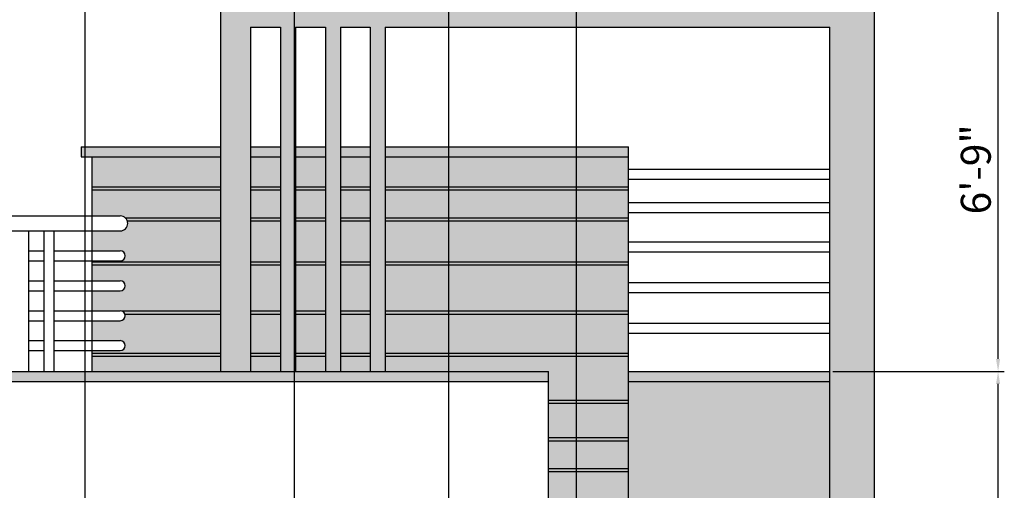
# Model space of a CAD drawing. Units: millimetres. Extents: x 4237 to 5109, y 21391 to 22486.
# Tile 4 of 17: x 4911 to 5109, y 21704 to 21798. Entities that reach past the tile are written whole.
import ezdxf

# ---------------------------------------------------------------- set-up
doc = ezdxf.new("R2010")
doc.units = ezdxf.units.MM
for name, color, linetype, lineweight in [('A-ANNO-DIMS', 2, 'Continuous', 18), ('A-ELEV', 7, 'Continuous', 25), ('A-ELEV-PATT', 252, 'Continuous', 13)]:
    doc.layers.add(name, color=color, linetype=linetype, lineweight=lineweight)
doc.styles.get("Standard").update_dxf_attribs({"font": 'arial.ttf'})
doc.dimstyles.new('ISO-25', dxfattribs={"dimtxt": 6, "dimasz": 2.5, "dimexe": 1.25, "dimexo": 0.625, "dimtad": 1, "dimdec": 1, "dimlunit": 4, "dimtxsty": 'Standard', "dimcen": 2.5, "dimadec": 0, "dimazin": 0, "dimtfac": 1, "dimtdec": 1, "dimtmove": 0, "dimatfit": 3, "dimfxl": 1, "dimarcsym": 0})

# ---------------------------------------------------------------- blocks, each defined once
blk = doc.blocks.new('*D130')
at = {"layer": 'A-ANNO-DIMS', "color": 0, "lineweight": -2, "transparency": 16777216}
for p, q in [((4878.54, 21688.54), (4878.54, 21897.84)), ((4881.04, 21896.59), (4921.78, 21896.59)), ((4924.28, 21686.68), (4924.28, 21897.84))]:
    blk.add_line(p, q, dxfattribs=at)
at = {"layer": 'A-ANNO-DIMS', "color": 0, "transparency": 16777216}
for points in [[(4881.04, 21897), (4881.04, 21896.17), (4878.54, 21896.59)], [(4921.78, 21897), (4921.78, 21896.17), (4924.28, 21896.59)]]:
    blk.add_solid(points, dxfattribs=at)
at = {"layer": 'Defpoints', "color": 0, "transparency": 16777216}
for p in [(4924.28, 21896.59), (4878.54, 21687.91), (4924.28, 21686.05)]:
    blk.add_point(p, dxfattribs=at)
at = {"layer": 'A-ANNO-DIMS', "color": 0, "transparency": 16777216, "insert": (4901.41, 21900.32), "char_height": 6, "attachment_point": 5}
blk.add_mtext('3\'-9 1/2"', dxfattribs=at)
blk = doc.blocks.new('*D131')
at = {"layer": 'A-ANNO-DIMS', "color": 0, "lineweight": -2, "transparency": 16777216}
for p, q in [((4924.28, 21686.68), (4924.28, 21897.84)), ((4926.78, 21896.59), (4963.73, 21896.59)), ((4966.23, 21686.68), (4966.23, 21897.84))]:
    blk.add_line(p, q, dxfattribs=at)
at = {"layer": 'A-ANNO-DIMS', "color": 0, "transparency": 16777216}
for points in [[(4926.78, 21897), (4926.78, 21896.17), (4924.28, 21896.59)], [(4963.73, 21897), (4963.73, 21896.17), (4966.23, 21896.59)]]:
    blk.add_solid(points, dxfattribs=at)
at = {"layer": 'Defpoints', "color": 0, "transparency": 16777216}
for p in [(4966.23, 21896.59), (4924.28, 21686.05), (4966.23, 21686.05)]:
    blk.add_point(p, dxfattribs=at)
at = {"layer": 'A-ANNO-DIMS', "color": 0, "transparency": 16777216, "insert": (4945.25, 21900.28), "char_height": 6, "attachment_point": 5}
blk.add_mtext('3\'-6"', dxfattribs=at)
blk = doc.blocks.new('*D132')
at = {"layer": 'A-ANNO-DIMS', "color": 0, "lineweight": -2, "transparency": 16777216}
for p, q in [((4966.23, 21686.68), (4966.23, 21897.84)), ((4968.73, 21896.59), (4994.7, 21896.59)), ((4997.2, 21689.78), (4997.2, 21897.84))]:
    blk.add_line(p, q, dxfattribs=at)
at = {"layer": 'A-ANNO-DIMS', "color": 0, "transparency": 16777216}
for points in [[(4968.73, 21897), (4968.73, 21896.17), (4966.23, 21896.59)], [(4994.7, 21897), (4994.7, 21896.17), (4997.2, 21896.59)]]:
    blk.add_solid(points, dxfattribs=at)
at = {"layer": 'Defpoints', "color": 0, "transparency": 16777216}
for p in [(4997.2, 21896.59), (4997.2, 21689.16), (4966.23, 21686.05)]:
    blk.add_point(p, dxfattribs=at)
at = {"layer": 'A-ANNO-DIMS', "color": 0, "transparency": 16777216, "insert": (4981.72, 21900.22), "char_height": 6, "attachment_point": 5}
blk.add_mtext('2\'-7"', dxfattribs=at)
blk = doc.blocks.new('*D133')
at = {"layer": 'A-ANNO-DIMS', "color": 0, "lineweight": -2, "transparency": 16777216}
for p, q in [((4997.2, 21689.78), (4997.2, 21897.84)), ((4999.7, 21896.59), (5020.26, 21896.59)), ((5022.76, 21689.78), (5022.76, 21897.84)), ((5022.76, 21896.59), (5056.55, 21896.59))]:
    blk.add_line(p, q, dxfattribs=at)
at = {"layer": 'A-ANNO-DIMS', "color": 0, "transparency": 16777216}
for points in [[(4999.7, 21897), (4999.7, 21896.17), (4997.2, 21896.59)], [(5020.26, 21897), (5020.26, 21896.17), (5022.76, 21896.59)]]:
    blk.add_solid(points, dxfattribs=at)
at = {"layer": 'Defpoints', "color": 0, "transparency": 16777216}
for p in [(5022.76, 21896.59), (4997.2, 21689.16), (5022.76, 21689.16)]:
    blk.add_point(p, dxfattribs=at)
at = {"layer": 'A-ANNO-DIMS', "color": 0, "transparency": 16777216, "insert": (5040.91, 21900.31), "char_height": 6, "attachment_point": 5}
blk.add_mtext('2\'-1 1/2"', dxfattribs=at)
blk = doc.blocks.new('*D134')
at = {"layer": 'A-ANNO-DIMS', "color": 0, "lineweight": -2, "transparency": 16777216}
for p, q in [((5022.76, 21689.78), (5022.76, 21897.84)), ((5025.26, 21896.59), (5080.03, 21896.59)), ((5082.53, 21809.46), (5082.53, 21897.84))]:
    blk.add_line(p, q, dxfattribs=at)
at = {"layer": 'A-ANNO-DIMS', "color": 0, "transparency": 16777216}
for points in [[(5025.26, 21897), (5025.26, 21896.17), (5022.76, 21896.59)], [(5080.03, 21897), (5080.03, 21896.17), (5082.53, 21896.59)]]:
    blk.add_solid(points, dxfattribs=at)
at = {"layer": 'Defpoints', "color": 0, "transparency": 16777216}
for p in [(5082.53, 21896.59), (5082.53, 21808.84), (5022.76, 21689.16)]:
    blk.add_point(p, dxfattribs=at)
at = {"layer": 'A-ANNO-DIMS', "color": 0, "transparency": 16777216, "insert": (5052.65, 21900.27), "char_height": 6, "attachment_point": 5}
blk.add_mtext('5\'-0"', dxfattribs=at)
blk = doc.blocks.new('*D136')
at = {"layer": 'A-ANNO-DIMS', "color": 0, "lineweight": -2, "transparency": 16777216}
for p, q in [((5074.15, 21727.84), (5108.53, 21727.84)), ((5107.28, 21560.34), (5107.28, 21725.34)), ((5083.15, 21557.84), (5108.53, 21557.84))]:
    blk.add_line(p, q, dxfattribs=at)
at = {"layer": 'A-ANNO-DIMS', "color": 0, "transparency": 16777216}
for points in [[(5106.86, 21725.34), (5107.69, 21725.34), (5107.28, 21727.84)], [(5106.86, 21560.34), (5107.69, 21560.34), (5107.28, 21557.84)]]:
    blk.add_solid(points, dxfattribs=at)
at = {"layer": 'Defpoints', "color": 0, "transparency": 16777216}
for p in [(5073.53, 21727.84), (5107.28, 21727.84), (5082.53, 21557.84)]:
    blk.add_point(p, dxfattribs=at)
at = {"layer": 'A-ANNO-DIMS', "color": 0, "transparency": 16777216, "insert": (5103.64, 21642.84), "char_height": 6, "attachment_point": 5, "rotation": 90}
blk.add_mtext('14\'-2"', dxfattribs=at)
blk = doc.blocks.new('*D137')
at = {"layer": 'A-ANNO-DIMS', "color": 0, "lineweight": -2, "transparency": 16777216}
for p, q in [((5083.15, 21808.84), (5108.53, 21808.84)), ((5107.28, 21730.34), (5107.28, 21806.34)), ((5074.15, 21727.84), (5108.53, 21727.84))]:
    blk.add_line(p, q, dxfattribs=at)
at = {"layer": 'A-ANNO-DIMS', "color": 0, "transparency": 16777216}
for points in [[(5106.86, 21806.34), (5107.69, 21806.34), (5107.28, 21808.84)], [(5106.86, 21730.34), (5107.69, 21730.34), (5107.28, 21727.84)]]:
    blk.add_solid(points, dxfattribs=at)
at = {"layer": 'Defpoints', "color": 0, "transparency": 16777216}
for p in [(5082.53, 21808.84), (5107.28, 21808.84), (5073.53, 21727.84)]:
    blk.add_point(p, dxfattribs=at)
at = {"layer": 'A-ANNO-DIMS', "color": 0, "transparency": 16777216, "insert": (5103.59, 21768.34), "char_height": 6, "attachment_point": 5, "rotation": 90}
blk.add_mtext('6\'-9"', dxfattribs=at)

msp = doc.modelspace()

# ---------------------------------------------------------------- hatches: boundary and pattern name
at = {"layer": 'A-ELEV-PATT'}
h = msp.add_hatch(color=256, dxfattribs=at)
h.dxf.hatch_style = 1
h.paths.add_polyline_path([(4957.45, 21796.84), (4963.45, 21796.84), (4963.45, 21727.84), (4966.45, 21727.84), (4966.45, 21796.84), (4972.45, 21796.84), (4972.45, 21727.84), (4975.45, 21727.84), (4975.45, 21796.84), (4981.45, 21796.84), (4981.45, 21727.84), (4984.45, 21727.84), (4984.45, 21796.84), (5073.53, 21796.84), (5073.53, 21557.84), (5082.53, 21557.84), (5082.53, 21808.84), (4951.45, 21808.84), (4951.45, 21727.84), (4957.45, 21727.84)])
h = msp.add_hatch(color=256, dxfattribs=at)
h.dxf.hatch_style = 1
h.paths.add_polyline_path([(4951.45, 21772.84), (4923.48, 21772.84), (4923.48, 21770.84), (4951.45, 21770.84)])
h = msp.add_hatch(color=256, dxfattribs=at)
h.dxf.hatch_style = 1
h.paths.add_polyline_path([(4963.45, 21772.84), (4957.45, 21772.84), (4957.45, 21770.84), (4963.45, 21770.84)])
h = msp.add_hatch(color=256, dxfattribs=at)
h.dxf.hatch_style = 1
h.paths.add_polyline_path([(4972.45, 21772.84), (4966.45, 21772.84), (4966.45, 21770.84), (4972.45, 21770.84)])
h = msp.add_hatch(color=256, dxfattribs=at)
h.dxf.hatch_style = 1
h.paths.add_polyline_path([(4981.45, 21772.84), (4975.45, 21772.84), (4975.45, 21770.84), (4981.45, 21770.84)])
h = msp.add_hatch(color=256, dxfattribs=at)
h.dxf.hatch_style = 1
h.paths.add_polyline_path([(5033.17, 21772.84), (4984.45, 21772.84), (4984.45, 21770.84), (5033.17, 21770.84)])
h = msp.add_hatch(color=256, dxfattribs=at)
h.dxf.hatch_style = 1
h.paths.add_polyline_path([(4951.45, 21770.84), (4925.69, 21770.84), (4925.69, 21764.85), (4951.45, 21764.85)])
h = msp.add_hatch(color=256, dxfattribs=at)
h.dxf.hatch_style = 1
h.paths.add_polyline_path([(4963.45, 21770.84), (4957.45, 21770.84), (4957.45, 21764.85), (4963.45, 21764.85)])
h = msp.add_hatch(color=256, dxfattribs=at)
h.dxf.hatch_style = 1
h.paths.add_polyline_path([(4972.45, 21770.84), (4966.45, 21770.84), (4966.45, 21764.85), (4972.45, 21764.85)])
h = msp.add_hatch(color=256, dxfattribs=at)
h.dxf.hatch_style = 1
h.paths.add_polyline_path([(4981.45, 21770.84), (4975.45, 21770.84), (4975.45, 21764.85), (4981.45, 21764.85)])
h = msp.add_hatch(color=256, dxfattribs=at)
h.dxf.hatch_style = 1
h.paths.add_polyline_path([(5033.17, 21770.84), (4984.45, 21770.84), (4984.45, 21764.85), (5033.17, 21764.85)])
h = msp.add_hatch(color=256, dxfattribs=at)
h.dxf.hatch_style = 1
h.paths.add_polyline_path([(4951.45, 21764.85), (4925.69, 21764.85), (4925.69, 21764.23), (4951.45, 21764.23)])
h = msp.add_hatch(color=256, dxfattribs=at)
h.dxf.hatch_style = 1
h.paths.add_polyline_path([(4951.45, 21764.23), (4925.69, 21764.23), (4925.69, 21759.01), (4931.32, 21759.01, -0.184847), (4932.32, 21758.63), (4951.45, 21758.63)])
h = msp.add_hatch(color=256, dxfattribs=at)
h.dxf.hatch_style = 1
h.paths.add_polyline_path([(4963.45, 21764.85), (4957.45, 21764.85), (4957.45, 21764.23), (4963.45, 21764.23)])
h = msp.add_hatch(color=256, dxfattribs=at)
h.dxf.hatch_style = 1
h.paths.add_polyline_path([(4963.45, 21764.23), (4957.45, 21764.23), (4957.45, 21758.63), (4963.45, 21758.63)])
h = msp.add_hatch(color=256, dxfattribs=at)
h.dxf.hatch_style = 1
h.paths.add_polyline_path([(4972.45, 21764.85), (4966.45, 21764.85), (4966.45, 21764.23), (4972.45, 21764.23)])
h = msp.add_hatch(color=256, dxfattribs=at)
h.dxf.hatch_style = 1
h.paths.add_polyline_path([(4972.45, 21764.23), (4966.45, 21764.23), (4966.45, 21758.63), (4972.45, 21758.63)])
h = msp.add_hatch(color=256, dxfattribs=at)
h.dxf.hatch_style = 1
h.paths.add_polyline_path([(4981.45, 21764.85), (4975.45, 21764.85), (4975.45, 21764.23), (4981.45, 21764.23)])
h = msp.add_hatch(color=256, dxfattribs=at)
h.dxf.hatch_style = 1
h.paths.add_polyline_path([(4981.45, 21764.23), (4975.45, 21764.23), (4975.45, 21758.63), (4981.45, 21758.63)])
h = msp.add_hatch(color=256, dxfattribs=at)
h.dxf.hatch_style = 1
h.paths.add_polyline_path([(5033.17, 21764.85), (4984.45, 21764.85), (4984.45, 21764.23), (5033.17, 21764.23)])
h = msp.add_hatch(color=256, dxfattribs=at)
h.dxf.hatch_style = 1
h.paths.add_polyline_path([(5033.17, 21764.23), (4984.45, 21764.23), (4984.45, 21758.63), (5033.17, 21758.63)])
h = msp.add_hatch(color=256, dxfattribs=at)
h.dxf.hatch_style = 1
h.paths.add_polyline_path([(4951.45, 21758.63), (4932.32, 21758.63, -0.127629), (4932.74, 21758), (4951.45, 21758)])
h = msp.add_hatch(color=256, dxfattribs=at)
h.dxf.hatch_style = 1
h.paths.add_polyline_path([(4963.45, 21758.63), (4957.45, 21758.63), (4957.45, 21758), (4963.45, 21758)])
h = msp.add_hatch(color=256, dxfattribs=at)
h.dxf.hatch_style = 1
h.paths.add_polyline_path([(4972.45, 21758.63), (4966.45, 21758.63), (4966.45, 21758), (4972.45, 21758)])
h = msp.add_hatch(color=256, dxfattribs=at)
h.dxf.hatch_style = 1
h.paths.add_polyline_path([(4981.45, 21758.63), (4975.45, 21758.63), (4975.45, 21758), (4981.45, 21758)])
h = msp.add_hatch(color=256, dxfattribs=at)
h.dxf.hatch_style = 1
h.paths.add_polyline_path([(5033.17, 21758.63), (4984.45, 21758.63), (4984.45, 21758), (5033.17, 21758)])
h = msp.add_hatch(color=256, dxfattribs=at)
h.dxf.hatch_style = 1
h.paths.add_polyline_path([(4951.45, 21758), (4932.74, 21758, -0.515121), (4931.32, 21756.01), (4925.69, 21756.01), (4925.69, 21752.01), (4931.32, 21752.01, -1), (4931.32, 21750.01), (4925.69, 21750.01), (4925.69, 21749.81), (4951.45, 21749.81)])
h = msp.add_hatch(color=256, dxfattribs=at)
h.dxf.hatch_style = 1
h.paths.add_polyline_path([(4963.45, 21758), (4957.45, 21758), (4957.45, 21749.81), (4963.45, 21749.81)])
h = msp.add_hatch(color=256, dxfattribs=at)
h.dxf.hatch_style = 1
h.paths.add_polyline_path([(4972.45, 21758), (4966.45, 21758), (4966.45, 21749.81), (4972.45, 21749.81)])
h = msp.add_hatch(color=256, dxfattribs=at)
h.dxf.hatch_style = 1
h.paths.add_polyline_path([(4981.45, 21758), (4975.45, 21758), (4975.45, 21749.81), (4981.45, 21749.81)])
h = msp.add_hatch(color=256, dxfattribs=at)
h.dxf.hatch_style = 1
h.paths.add_polyline_path([(5033.17, 21758), (4984.45, 21758), (4984.45, 21749.81), (5033.17, 21749.81)])
h = msp.add_hatch(color=256, dxfattribs=at)
h.dxf.hatch_style = 1
h.paths.add_polyline_path([(4951.45, 21749.81), (4925.69, 21749.81), (4925.69, 21749.18), (4951.45, 21749.18)])
h = msp.add_hatch(color=256, dxfattribs=at)
h.dxf.hatch_style = 1
h.paths.add_polyline_path([(4951.45, 21749.18), (4925.69, 21749.18), (4925.69, 21746.01), (4931.32, 21746.01, -1), (4931.32, 21744.01), (4925.69, 21744.01), (4925.69, 21740.01), (4931.32, 21740.01, -0.068465), (4931.59, 21739.97), (4951.45, 21739.97)])
h = msp.add_hatch(color=256, dxfattribs=at)
h.dxf.hatch_style = 1
h.paths.add_polyline_path([(4963.45, 21749.81), (4957.45, 21749.81), (4957.45, 21749.18), (4963.45, 21749.18)])
h = msp.add_hatch(color=256, dxfattribs=at)
h.dxf.hatch_style = 1
h.paths.add_polyline_path([(4963.45, 21749.18), (4957.45, 21749.18), (4957.45, 21739.97), (4963.45, 21739.97)])
h = msp.add_hatch(color=256, dxfattribs=at)
h.dxf.hatch_style = 1
h.paths.add_polyline_path([(4972.45, 21749.81), (4966.45, 21749.81), (4966.45, 21749.18), (4972.45, 21749.18)])
h = msp.add_hatch(color=256, dxfattribs=at)
h.dxf.hatch_style = 1
h.paths.add_polyline_path([(4972.45, 21749.18), (4966.45, 21749.18), (4966.45, 21739.97), (4972.45, 21739.97)])
h = msp.add_hatch(color=256, dxfattribs=at)
h.dxf.hatch_style = 1
h.paths.add_polyline_path([(4981.45, 21749.81), (4975.45, 21749.81), (4975.45, 21749.18), (4981.45, 21749.18)])
h = msp.add_hatch(color=256, dxfattribs=at)
h.dxf.hatch_style = 1
h.paths.add_polyline_path([(4981.45, 21749.18), (4975.45, 21749.18), (4975.45, 21739.97), (4981.45, 21739.97)])
h = msp.add_hatch(color=256, dxfattribs=at)
h.dxf.hatch_style = 1
h.paths.add_polyline_path([(5033.17, 21749.81), (4984.45, 21749.81), (4984.45, 21749.18), (5033.17, 21749.18)])
h = msp.add_hatch(color=256, dxfattribs=at)
h.dxf.hatch_style = 1
h.paths.add_polyline_path([(5033.17, 21749.18), (4984.45, 21749.18), (4984.45, 21739.97), (5033.17, 21739.97)])
h = msp.add_hatch(color=256, dxfattribs=at)
h.dxf.hatch_style = 1
h.paths.add_polyline_path([(4951.45, 21739.34), (4932.26, 21739.34, -0.518188), (4931.32, 21738.01), (4925.69, 21738.01), (4925.69, 21734.01), (4931.32, 21734.01, -1), (4931.32, 21732.01), (4925.69, 21732.01), (4925.69, 21731.53), (4951.45, 21731.53)])
h = msp.add_hatch(color=256, dxfattribs=at)
h.dxf.hatch_style = 1
h.paths.add_polyline_path([(4951.45, 21739.97), (4931.59, 21739.97, -0.243601), (4932.26, 21739.34), (4951.45, 21739.34)])
h = msp.add_hatch(color=256, dxfattribs=at)
h.dxf.hatch_style = 1
h.paths.add_polyline_path([(4963.45, 21739.97), (4957.45, 21739.97), (4957.45, 21739.34), (4963.45, 21739.34)])
h = msp.add_hatch(color=256, dxfattribs=at)
h.dxf.hatch_style = 1
h.paths.add_polyline_path([(4963.45, 21739.34), (4957.45, 21739.34), (4957.45, 21731.53), (4963.45, 21731.53)])
h = msp.add_hatch(color=256, dxfattribs=at)
h.dxf.hatch_style = 1
h.paths.add_polyline_path([(4972.45, 21739.97), (4966.45, 21739.97), (4966.45, 21739.34), (4972.45, 21739.34)])
h = msp.add_hatch(color=256, dxfattribs=at)
h.dxf.hatch_style = 1
h.paths.add_polyline_path([(4972.45, 21739.34), (4966.45, 21739.34), (4966.45, 21731.53), (4972.45, 21731.53)])
h = msp.add_hatch(color=256, dxfattribs=at)
h.dxf.hatch_style = 1
h.paths.add_polyline_path([(4981.45, 21739.97), (4975.45, 21739.97), (4975.45, 21739.34), (4981.45, 21739.34)])
h = msp.add_hatch(color=256, dxfattribs=at)
h.dxf.hatch_style = 1
h.paths.add_polyline_path([(4981.45, 21739.34), (4975.45, 21739.34), (4975.45, 21731.53), (4981.45, 21731.53)])
h = msp.add_hatch(color=256, dxfattribs=at)
h.dxf.hatch_style = 1
h.paths.add_polyline_path([(5033.17, 21739.97), (4984.45, 21739.97), (4984.45, 21739.34), (5033.17, 21739.34)])
h = msp.add_hatch(color=256, dxfattribs=at)
h.dxf.hatch_style = 1
h.paths.add_polyline_path([(5033.17, 21739.34), (4984.45, 21739.34), (4984.45, 21731.53), (5033.17, 21731.53)])
h = msp.add_hatch(color=256, dxfattribs=at)
h.dxf.hatch_style = 1
h.paths.add_polyline_path([(4951.45, 21731.53), (4925.69, 21731.53), (4925.69, 21730.91), (4951.45, 21730.91)])
h = msp.add_hatch(color=256, dxfattribs=at)
h.dxf.hatch_style = 1
h.paths.add_polyline_path([(4951.45, 21730.91), (4925.69, 21730.91), (4925.69, 21727.84), (4951.45, 21727.84)])
h = msp.add_hatch(color=256, dxfattribs=at)
h.dxf.hatch_style = 1
h.paths.add_polyline_path([(4963.45, 21731.53), (4957.45, 21731.53), (4957.45, 21730.91), (4963.45, 21730.91)])
h = msp.add_hatch(color=256, dxfattribs=at)
h.dxf.hatch_style = 1
h.paths.add_polyline_path([(4963.45, 21730.91), (4957.45, 21730.91), (4957.45, 21727.84), (4963.45, 21727.84)])
h = msp.add_hatch(color=256, dxfattribs=at)
h.dxf.hatch_style = 1
h.paths.add_polyline_path([(4972.45, 21731.53), (4966.45, 21731.53), (4966.45, 21730.91), (4972.45, 21730.91)])
h = msp.add_hatch(color=256, dxfattribs=at)
h.dxf.hatch_style = 1
h.paths.add_polyline_path([(4972.45, 21730.91), (4966.45, 21730.91), (4966.45, 21727.84), (4972.45, 21727.84)])
h = msp.add_hatch(color=256, dxfattribs=at)
h.dxf.hatch_style = 1
h.paths.add_polyline_path([(4981.45, 21731.53), (4975.45, 21731.53), (4975.45, 21730.91), (4981.45, 21730.91)])
h = msp.add_hatch(color=256, dxfattribs=at)
h.dxf.hatch_style = 1
h.paths.add_polyline_path([(4981.45, 21730.91), (4975.45, 21730.91), (4975.45, 21727.84), (4981.45, 21727.84)])
h = msp.add_hatch(color=256, dxfattribs=at)
h.dxf.hatch_style = 1
h.paths.add_polyline_path([(5033.17, 21731.53), (4984.45, 21731.53), (4984.45, 21730.91), (5033.17, 21730.91)])
h = msp.add_hatch(color=256, dxfattribs=at)
h.dxf.hatch_style = 1
h.paths.add_polyline_path([(5033.17, 21730.91), (4984.45, 21730.91), (4984.45, 21727.84), (5017.14, 21727.84), (5017.14, 21722.08), (5033.17, 21722.08)])
h = msp.add_hatch(color=256, dxfattribs=at)
h.dxf.hatch_style = 1
h.paths.add_polyline_path([(5017.14, 21727.84), (4742.84, 21727.84), (4742.84, 21725.84), (5017.14, 21725.84)])
h = msp.add_hatch(color=256, dxfattribs=at)
h.dxf.hatch_style = 1
h.paths.add_polyline_path([(5073.53, 21727.84), (5033.17, 21727.84), (5033.17, 21725.84), (5073.53, 21725.84)])
h = msp.add_hatch(color=256, dxfattribs=at)
h.dxf.hatch_style = 1
h.paths.add_polyline_path([(5073.53, 21725.84), (5033.17, 21725.84), (5033.17, 21557.84), (5073.53, 21557.84)])
h = msp.add_hatch(color=256, dxfattribs=at)
h.dxf.hatch_style = 1
h.paths.add_polyline_path([(5033.17, 21722.08), (5017.14, 21722.08), (5017.14, 21721.45), (5033.17, 21721.45)])
h = msp.add_hatch(color=256, dxfattribs=at)
h.dxf.hatch_style = 1
h.paths.add_polyline_path([(5033.17, 21721.45), (5017.14, 21721.45), (5017.14, 21714.57), (5033.17, 21714.57)])
h = msp.add_hatch(color=256, dxfattribs=at)
h.dxf.hatch_style = 1
h.paths.add_polyline_path([(5033.17, 21714.57), (5017.14, 21714.57), (5017.14, 21713.94), (5033.17, 21713.94)])
h = msp.add_hatch(color=256, dxfattribs=at)
h.dxf.hatch_style = 1
h.paths.add_polyline_path([(5033.17, 21713.94), (5017.14, 21713.94), (5017.14, 21708.38), (5033.17, 21708.38)])
h = msp.add_hatch(color=256, dxfattribs=at)
h.dxf.hatch_style = 1
h.paths.add_polyline_path([(5033.17, 21707.76), (5017.14, 21707.76), (5017.14, 21701.84), (5013.1, 21701.84), (5013.1, 21699.14), (5033.17, 21699.14)])
h = msp.add_hatch(color=256, dxfattribs=at)
h.dxf.hatch_style = 1
h.paths.add_polyline_path([(5033.17, 21708.38), (5017.14, 21708.38), (5017.14, 21707.76), (5033.17, 21707.76)])

# ---------------------------------------------------------------- linework, layer by layer
at = {"layer": 'A-ELEV'}
for p, q in [((4951.45, 21808.84), (4951.45, 21727.84)), ((5082.53, 21425.84), (5082.53, 21808.84)), ((4957.45, 21796.84), (4963.45, 21796.84)), ((4957.45, 21796.84), (4957.45, 21727.84)), ((4963.45, 21796.84), (4963.45, 21727.84)), ((4966.45, 21796.84), (4972.45, 21796.84)), ((4966.45, 21796.84), (4966.45, 21727.84)), ((4972.45, 21796.84), (4972.45, 21727.84)), ((4975.45, 21796.84), (4981.45, 21796.84)), ((4975.45, 21796.84), (4975.45, 21727.84)), ((4981.45, 21796.84), (4981.45, 21727.84)), ((4984.45, 21796.84), (5073.53, 21796.84)), ((4984.45, 21796.84), (4984.45, 21727.84)), ((5073.53, 21425.84), (5073.53, 21796.84)), ((4923.48, 21772.84), (4951.45, 21772.84)), ((4923.48, 21772.84), (4923.48, 21770.84)), ((4957.45, 21772.84), (4963.45, 21772.84)), ((4966.45, 21772.84), (4972.45, 21772.84)), ((4975.45, 21772.84), (4981.45, 21772.84)), ((4984.45, 21772.84), (5033.17, 21772.84)), ((5033.17, 21557.84), (5033.17, 21772.84)), ((4923.48, 21770.84), (4951.45, 21770.84)), ((4925.69, 21727.84), (4925.69, 21770.84)), ((4957.45, 21770.84), (4963.45, 21770.84)), ((4966.45, 21770.84), (4972.45, 21770.84)), ((4975.45, 21770.84), (4981.45, 21770.84)), ((4984.45, 21770.84), (5033.17, 21770.84)), ((5033.17, 21768.36), (5073.53, 21768.36)), ((5033.17, 21766.36), (5073.53, 21766.36)), ((4925.69, 21764.85), (4951.45, 21764.85)), ((4925.69, 21764.23), (4951.45, 21764.23)), ((4957.45, 21764.85), (4963.45, 21764.85)), ((4957.45, 21764.23), (4963.45, 21764.23)), ((4966.45, 21764.85), (4972.45, 21764.85)), ((4966.45, 21764.23), (4972.45, 21764.23)), ((4975.45, 21764.85), (4981.45, 21764.85)), ((4975.45, 21764.23), (4981.45, 21764.23)), ((4984.45, 21764.85), (5033.17, 21764.85)), ((4984.45, 21764.23), (5033.17, 21764.23)), ((5033.17, 21761.67), (5073.53, 21761.67)), ((4817.54, 21759.01), (4931.32, 21759.01)), ((4932.32, 21758.63), (4951.45, 21758.63)), ((4957.45, 21758.63), (4963.45, 21758.63)), ((4966.45, 21758.63), (4972.45, 21758.63)), ((4975.45, 21758.63), (4981.45, 21758.63)), ((4984.45, 21758.63), (5033.17, 21758.63)), ((5033.17, 21759.67), (5073.53, 21759.67)), ((4932.74, 21758), (4951.45, 21758)), ((4957.45, 21758), (4963.45, 21758)), ((4966.45, 21758), (4972.45, 21758)), ((4975.45, 21758), (4981.45, 21758)), ((4984.45, 21758), (5033.17, 21758)), ((4817.54, 21756.01), (4931.32, 21756.01)), ((4912.97, 21756.01), (4912.97, 21727.84)), ((4916.01, 21756.01), (4916.01, 21727.84)), ((4918.01, 21756.01), (4918.01, 21727.84)), ((5033.17, 21753.81), (5073.53, 21753.81)), ((4912.97, 21752.01), (4916.01, 21752.01)), ((4918.01, 21752.01), (4931.32, 21752.01)), ((5033.17, 21751.81), (5073.53, 21751.81)), ((4912.97, 21750.01), (4916.01, 21750.01)), ((4918.01, 21750.01), (4931.32, 21750.01)), ((4925.69, 21749.81), (4951.45, 21749.81)), ((4925.69, 21749.18), (4951.45, 21749.18)), ((4957.45, 21749.81), (4963.45, 21749.81)), ((4957.45, 21749.18), (4963.45, 21749.18)), ((4966.45, 21749.81), (4972.45, 21749.81)), ((4966.45, 21749.18), (4972.45, 21749.18)), ((4975.45, 21749.81), (4981.45, 21749.81)), ((4975.45, 21749.18), (4981.45, 21749.18)), ((4984.45, 21749.81), (5033.17, 21749.81)), ((4984.45, 21749.18), (5033.17, 21749.18)), ((4912.97, 21746.01), (4916.01, 21746.01)), ((4918.01, 21746.01), (4931.32, 21746.01)), ((5033.17, 21745.66), (5073.53, 21745.66)), ((4912.97, 21744.01), (4916.01, 21744.01)), ((4918.01, 21744.01), (4931.32, 21744.01)), ((5033.17, 21743.66), (5073.53, 21743.66)), ((4912.97, 21740.01), (4916.01, 21740.01)), ((4918.01, 21740.01), (4931.32, 21740.01)), ((4931.59, 21739.97), (4951.45, 21739.97)), ((4932.26, 21739.34), (4951.45, 21739.34)), ((4957.45, 21739.97), (4963.45, 21739.97)), ((4957.45, 21739.34), (4963.45, 21739.34)), ((4966.45, 21739.97), (4972.45, 21739.97)), ((4966.45, 21739.34), (4972.45, 21739.34)), ((4975.45, 21739.97), (4981.45, 21739.97)), ((4975.45, 21739.34), (4981.45, 21739.34)), ((4984.45, 21739.97), (5033.17, 21739.97)), ((4984.45, 21739.34), (5033.17, 21739.34)), ((4912.97, 21738.01), (4916.01, 21738.01)), ((4918.01, 21738.01), (4931.32, 21738.01)), ((5033.17, 21737.51), (5073.53, 21737.51)), ((5033.17, 21735.51), (5073.53, 21735.51)), ((4912.97, 21734.01), (4916.01, 21734.01)), ((4918.01, 21734.01), (4931.32, 21734.01)), ((4912.97, 21732.01), (4916.01, 21732.01)), ((4918.01, 21732.01), (4931.32, 21732.01)), ((4925.69, 21731.53), (4951.45, 21731.53)), ((4925.69, 21730.91), (4951.45, 21730.91)), ((4957.45, 21731.53), (4963.45, 21731.53)), ((4957.45, 21730.91), (4963.45, 21730.91)), ((4966.45, 21731.53), (4972.45, 21731.53)), ((4966.45, 21730.91), (4972.45, 21730.91)), ((4975.45, 21731.53), (4981.45, 21731.53)), ((4975.45, 21730.91), (4981.45, 21730.91)), ((4984.45, 21731.53), (5033.17, 21731.53)), ((4984.45, 21730.91), (5033.17, 21730.91)), ((4742.84, 21727.84), (5017.14, 21727.84)), ((5017.14, 21701.84), (5017.14, 21727.84)), ((5033.17, 21727.84), (5073.53, 21727.84)), ((4742.84, 21725.84), (5017.14, 21725.84)), ((5033.17, 21725.84), (5073.53, 21725.84)), ((5017.14, 21722.08), (5033.17, 21722.08)), ((5017.14, 21721.45), (5033.17, 21721.45)), ((5017.14, 21714.57), (5033.17, 21714.57)), ((5017.14, 21713.94), (5033.17, 21713.94)), ((5017.14, 21708.38), (5033.17, 21708.38)), ((5017.14, 21707.76), (5033.17, 21707.76))]:
    msp.add_line(p, q, dxfattribs=at)
for centre, radius in [((4931.32, 21757.51), 1.5), ((4931.32, 21751.01), 1), ((4931.32, 21745.01), 1), ((4931.32, 21739.01), 1), ((4931.32, 21733.01), 1)]:
    msp.add_arc(centre, radius, 270, 90, dxfattribs=at)

# ---------------------------------------------------------------- dimensions: what is measured, and where the dimension line sits
at = {"layer": 'A-ANNO-DIMS'}
for base, p1, p2, picture, middle in [((4924.28, 21896.59), (4878.54, 21687.91), (4924.28, 21686.05), '*D130', (4901.41, 21900.32)), ((5022.76, 21896.59), (4997.2, 21689.16), (5022.76, 21689.16), '*D133', (5040.91, 21900.31)), ((4966.2267, 21896.586), (4924.2801, 21686.0515), (4966.2267, 21686.0515), '*D131', (4945.2534, 21900.2765)), ((4997.2, 21896.59), (4966.23, 21686.05), (4997.2, 21689.16), '*D132', (4981.72, 21900.22)), ((5082.53, 21896.59), (5022.76, 21689.16), (5082.53, 21808.84), '*D134', (5052.65, 21900.27))]:
    dim = msp.add_linear_dim(base=base, p1=p1, p2=p2, dimstyle='ISO-25', override={"dimdec": 1, "dimlfac": 1, "dimrnd": 0, "dimzin": 1, "dimdsep": 46, "dimlunit": 4, "dimfrac": 2}, dxfattribs=at)
    dim.commit()
    dim.dimension.update_dxf_attribs({"geometry": picture, "text_midpoint": middle})
for base, p1, p2, picture, middle in [((5107.28, 21808.84), (5073.53, 21727.84), (5082.53, 21808.84), '*D137', (5103.59, 21768.34)), ((5107.28, 21727.84), (5082.53, 21557.84), (5073.53, 21727.84), '*D136', (5103.64, 21642.84))]:
    dim = msp.add_linear_dim(base=base, p1=p1, p2=p2, angle=90, dimstyle='ISO-25', override={"dimdec": 1, "dimlfac": 1, "dimrnd": 0, "dimzin": 1, "dimdsep": 46, "dimlunit": 4, "dimfrac": 2}, dxfattribs=at)
    dim.commit()
    dim.dimension.update_dxf_attribs({"geometry": picture, "text_midpoint": middle})

doc.saveas('drawing.dxf')
